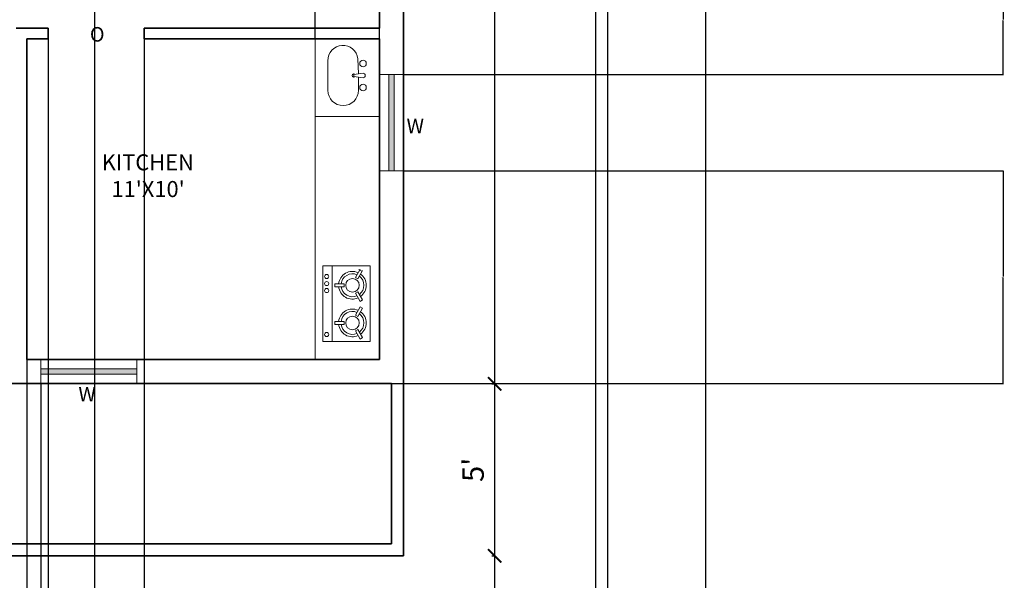
# Model space of a CAD drawing. Units: inches. Extents: x 502 to 1235, y -850 to 110.
# Tile 3 of 9: x 867 to 1235, y -625 to -415. Entities that reach past the tile are written whole.
import ezdxf

# ---------------------------------------------------------------- set-up
doc = ezdxf.new("R2010")
doc.units = ezdxf.units.IN
doc.header["$MEASUREMENT"] = 0
for name, color, linetype, lineweight in [('A-ANNO-DIMS', 2, 'Continuous', 18), ('A-ANNO-TEXT', 7, 'Continuous', 18), ('A-AREA-IDEN', 8, 'Continuous', 18), ('A-EQPM', 50, 'Continuous', 18), ('A-FLOR-CASE', 50, 'Continuous', 18), ('A-FLOR-FIXT', 50, 'Continuous', 18), ('A-GLAZ-PATT', 5, 'Continuous', 13), ('C-PROP', 1, 'Continuous', 25), ('WALL', 1, 'Continuous', 35), ('WIN', 5, 'Continuous', 18)]:
    doc.layers.add(name, color=color, linetype=linetype, lineweight=lineweight)
doc.styles.get("Standard").update_dxf_attribs({"font": 'arial.ttf'})
doc.dimstyles.get("Standard").update_dxf_attribs({"dimtxt": 0.18, "dimasz": 0.18, "dimexe": 0.18, "dimexo": 0.0625, "dimgap": 0.09, "dimtad": 0, "dimtih": 1, "dimtoh": 1, "dimdec": 1, "dimzin": 0, "dimdsep": 46, "dimlunit": 4, "dimtxsty": 'Standard', "dimcen": 0.09, "dimadec": 0, "dimazin": 0, "dimtfac": 1, "dimtdec": 1, "dimtofl": 0, "dimtmove": 0, "dimatfit": 3, "dimfxl": 1, "dimtolj": 1, "dimtzin": 0, "dimarcsym": 0})

# ---------------------------------------------------------------- blocks, each defined once
blk = doc.blocks.new('_ArchTick')
at = {"color": 0, "linetype": 'ByBlock', "const_width": 0.15}
blk.add_lwpolyline([(-0.5, -0.5), (0.5, 0.5)], dxfattribs=at)
blk = doc.blocks.new('*D6')
at = {"layer": 'A-ANNO-DIMS', "color": 0, "lineweight": -2, "transparency": 16777216}
for p, q in [((1122.49, 15.65), (1123.67, 15.65)), ((1123.49, 15.65), (1123.49, -704.35)), ((1122.49, -704.35), (1123.67, -704.35))]:
    blk.add_line(p, q, dxfattribs=at)
at = {"layer": 'Defpoints', "color": 0, "transparency": 16777216}
for p in [(1086.89, 15.65), (1086.89, -704.35), (1123.49, -704.35)]:
    blk.add_point(p, dxfattribs=at)
at = {"layer": 'A-ANNO-DIMS', "color": 0, "lineweight": -2, "transparency": 16777216, "xscale": 5, "yscale": 5, "zscale": 5}
for p, rotation in [((1123.49, 15.65), 90), ((1123.49, -704.35), 270)]:
    blk.add_blockref('_ArchTick', p, dxfattribs=dict(at, rotation=rotation))
at = {"layer": 'A-ANNO-DIMS', "color": 0, "transparency": 16777216, "insert": (1115.41, -344.35), "char_height": 8, "attachment_point": 5, "rotation": 90}
blk.add_mtext("\\A1;60'", dxfattribs=at)
blk = doc.blocks.new('*D7')
at = {"layer": 'A-ANNO-DIMS', "color": 0, "lineweight": -2, "transparency": 16777216}
for p, q in [((1043.54, -60.85), (1044.72, -60.85)), ((1044.54, -60.85), (1044.54, -551.48)), ((1043.54, -551.48), (1044.72, -551.48))]:
    blk.add_line(p, q, dxfattribs=at)
at = {"layer": 'Defpoints', "color": 0, "transparency": 16777216}
for p in [(1010.39, -60.85), (1010.39, -551.48), (1044.54, -551.48)]:
    blk.add_point(p, dxfattribs=at)
at = {"layer": 'A-ANNO-DIMS', "color": 0, "lineweight": -2, "transparency": 16777216, "xscale": 5, "yscale": 5, "zscale": 5}
for p, rotation in [((1044.54, -60.85), 90), ((1044.54, -551.48), 270)]:
    blk.add_blockref('_ArchTick', p, dxfattribs=dict(at, rotation=rotation))
at = {"layer": 'A-ANNO-DIMS', "color": 0, "transparency": 16777216, "insert": (1036.52, -306.16), "char_height": 8, "attachment_point": 5, "rotation": 90}
blk.add_mtext("\\A1;42'", dxfattribs=at)
blk = doc.blocks.new('*D8')
at = {"layer": 'A-ANNO-DIMS', "color": 0, "lineweight": -2, "transparency": 16777216}
for p, q in [((1043.54, -551.48), (1044.72, -551.48)), ((1044.54, -551.48), (1044.54, -615.85)), ((1043.54, -615.85), (1044.72, -615.85))]:
    blk.add_line(p, q, dxfattribs=at)
at = {"layer": 'Defpoints', "color": 0, "transparency": 16777216}
for p in [(1010.39, -551.48), (1010.39, -615.85), (1044.54, -615.85)]:
    blk.add_point(p, dxfattribs=at)
at = {"layer": 'A-ANNO-DIMS', "color": 0, "lineweight": -2, "transparency": 16777216, "xscale": 5, "yscale": 5, "zscale": 5}
for p, rotation in [((1044.54, -551.48), 90), ((1044.54, -615.85), 270)]:
    blk.add_blockref('_ArchTick', p, dxfattribs=dict(at, rotation=rotation))
at = {"layer": 'A-ANNO-DIMS', "color": 0, "transparency": 16777216, "insert": (1036.47, -583.66), "char_height": 8, "attachment_point": 5, "rotation": 90}
blk.add_mtext("\\A1;5'", dxfattribs=at)
blk = doc.blocks.new('*D9')
at = {"layer": 'A-ANNO-DIMS', "color": 0, "lineweight": -2, "transparency": 16777216}
for p, q in [((1043.54, -615.85), (1044.72, -615.85)), ((1044.54, -615.85), (1044.54, -699.85)), ((1043.54, -699.85), (1044.72, -699.85))]:
    blk.add_line(p, q, dxfattribs=at)
at = {"layer": 'Defpoints', "color": 0, "transparency": 16777216}
for p in [(1010.39, -615.85), (1012.7, -699.85), (1044.54, -699.85)]:
    blk.add_point(p, dxfattribs=at)
at = {"layer": 'A-ANNO-DIMS', "color": 0, "lineweight": -2, "transparency": 16777216, "xscale": 5, "yscale": 5, "zscale": 5}
for p, rotation in [((1044.54, -615.85), 90), ((1044.54, -699.85), 270)]:
    blk.add_blockref('_ArchTick', p, dxfattribs=dict(at, rotation=rotation))
at = {"layer": 'A-ANNO-DIMS', "color": 0, "transparency": 16777216, "insert": (1036.54, -657.85), "char_height": 8, "attachment_point": 5, "rotation": 90}
blk.add_mtext("\\A1;7'", dxfattribs=at)
blk = doc.blocks.new('WIN-36IN')
for p, q in [((0, 0), (0, 9)), ((36, 0), (36, 9)), ((0, 5.5), (36, 5.5)), ((0, 3.5), (36, 3.5))]:
    blk.add_line(p, q)
blk = doc.blocks.new('*D25')
at = {"layer": 'A-ANNO-DIMS', "color": 0, "lineweight": -2, "transparency": 16777216}
for p, q in [((798.89, -699.78), (798.89, 63.98)), ((799.07, 63.8), (846.56, 63.8)), ((894.71, 63.8), (847.22, 63.8)), ((894.89, -699.78), (894.89, 63.98))]:
    blk.add_line(p, q, dxfattribs=at)
at = {"layer": 'A-ANNO-DIMS', "color": 0, "transparency": 16777216}
for points in [[(799.07, 63.83), (799.07, 63.77), (798.89, 63.8)], [(894.71, 63.83), (894.71, 63.77), (894.89, 63.8)]]:
    blk.add_solid(points, dxfattribs=at)
at = {"layer": 'Defpoints', "color": 0, "transparency": 16777216}
for p in [(894.89, 63.8), (798.89, -699.85), (894.89, -699.85)]:
    blk.add_point(p, dxfattribs=at)
at = {"layer": 'A-ANNO-DIMS', "color": 0, "transparency": 16777216, "insert": (846.89, 63.8), "char_height": 0.18, "attachment_point": 5}
blk.add_mtext('\\A1;8\'-0"', dxfattribs=at)
blk = doc.blocks.new('*D41')
at = {"layer": 'A-ANNO-DIMS', "color": 0, "lineweight": -2, "transparency": 16777216}
for p, q in [((877.39, -422.41), (877.39, -844.7)), ((913.39, -422.41), (913.39, -844.7)), ((877.57, -844.52), (895.06, -844.52)), ((913.21, -844.52), (895.72, -844.52))]:
    blk.add_line(p, q, dxfattribs=at)
at = {"layer": 'A-ANNO-DIMS', "color": 0, "transparency": 16777216}
for points in [[(877.57, -844.49), (877.57, -844.55), (877.39, -844.52)], [(913.21, -844.49), (913.21, -844.55), (913.39, -844.52)]]:
    blk.add_solid(points, dxfattribs=at)
at = {"layer": 'Defpoints', "color": 0, "transparency": 16777216}
for p in [(877.39, -422.35), (913.39, -422.35), (913.39, -844.52)]:
    blk.add_point(p, dxfattribs=at)
at = {"layer": 'A-ANNO-DIMS', "color": 0, "transparency": 16777216, "insert": (895.39, -844.52), "char_height": 0.18, "attachment_point": 5}
blk.add_mtext('\\A1;3\'-0"', dxfattribs=at)
blk = doc.blocks.new('*D42')
at = {"layer": 'A-ANNO-DIMS', "color": 0, "lineweight": -2, "transparency": 16777216}
for p, q in [((869.39, -422.41), (869.39, -844.7)), ((877.39, -422.41), (877.39, -844.7)), ((869.57, -844.52), (873.06, -844.52)), ((877.21, -844.52), (873.72, -844.52))]:
    blk.add_line(p, q, dxfattribs=at)
at = {"layer": 'A-ANNO-DIMS', "color": 0, "transparency": 16777216}
for points in [[(869.57, -844.49), (869.57, -844.55), (869.39, -844.52)], [(877.21, -844.49), (877.21, -844.55), (877.39, -844.52)]]:
    blk.add_solid(points, dxfattribs=at)
at = {"layer": 'Defpoints', "color": 0, "transparency": 16777216}
for p in [(869.39, -422.35), (877.39, -422.35), (877.39, -844.52)]:
    blk.add_point(p, dxfattribs=at)
at = {"layer": 'A-ANNO-DIMS', "color": 0, "transparency": 16777216, "insert": (873.39, -844.52), "char_height": 0.18, "attachment_point": 5}
blk.add_mtext('\\A1;0\'-8"', dxfattribs=at)
blk = doc.blocks.new('*D43')
at = {"layer": 'A-ANNO-DIMS', "color": 0, "lineweight": -2, "transparency": 16777216}
for p, q in [((977.39, -422.28), (977.39, 63.98)), ((977.57, 63.8), (989.06, 63.8)), ((1001.21, 63.8), (989.72, 63.8)), ((1001.39, -422.28), (1001.39, 63.98))]:
    blk.add_line(p, q, dxfattribs=at)
at = {"layer": 'A-ANNO-DIMS', "color": 0, "transparency": 16777216}
for points in [[(977.57, 63.83), (977.57, 63.77), (977.39, 63.8)], [(1001.21, 63.83), (1001.21, 63.77), (1001.39, 63.8)]]:
    blk.add_solid(points, dxfattribs=at)
at = {"layer": 'Defpoints', "color": 0, "transparency": 16777216}
for p in [(1001.39, 63.8), (977.39, -422.35), (1001.39, -422.35)]:
    blk.add_point(p, dxfattribs=at)
at = {"layer": 'A-ANNO-DIMS', "color": 0, "transparency": 16777216, "insert": (989.39, 63.8), "char_height": 0.18, "attachment_point": 5}
blk.add_mtext('\\A1;2\'-0"', dxfattribs=at)
blk = doc.blocks.new('*D47')
at = {"layer": 'A-ANNO-DIMS', "color": 0, "lineweight": -2, "transparency": 16777216}
for p, q in [((857.39, -551.41), (857.39, -844.7)), ((874.64, -551.41), (874.64, -844.7)), ((857.57, -844.52), (865.69, -844.52)), ((874.46, -844.52), (866.34, -844.52))]:
    blk.add_line(p, q, dxfattribs=at)
at = {"layer": 'A-ANNO-DIMS', "color": 0, "transparency": 16777216}
for points in [[(857.57, -844.49), (857.57, -844.55), (857.39, -844.52)], [(874.46, -844.49), (874.46, -844.55), (874.64, -844.52)]]:
    blk.add_solid(points, dxfattribs=at)
at = {"layer": 'Defpoints', "color": 0, "transparency": 16777216}
for p in [(857.39, -551.35), (874.64, -551.35), (874.64, -844.52)]:
    blk.add_point(p, dxfattribs=at)
at = {"layer": 'A-ANNO-DIMS', "color": 0, "transparency": 16777216, "insert": (866.01, -844.52), "char_height": 0.18, "attachment_point": 5}
blk.add_mtext('\\A1;1\'-5"', dxfattribs=at)
blk = doc.blocks.new('*D54')
at = {"layer": 'A-ANNO-DIMS', "color": 0, "lineweight": -2, "transparency": 16777216}
for p, q in [((1010.45, -471.74), (1235.01, -471.74)), ((1234.83, -471.92), (1234.83, -511.36)), ((1234.83, -551.17), (1234.83, -511.73)), ((1005.95, -551.35), (1235.01, -551.35))]:
    blk.add_line(p, q, dxfattribs=at)
at = {"layer": 'A-ANNO-DIMS', "color": 0, "transparency": 16777216}
for points in [[(1234.8, -471.92), (1234.86, -471.92), (1234.83, -471.74)], [(1234.8, -551.17), (1234.86, -551.17), (1234.83, -551.35)]]:
    blk.add_solid(points, dxfattribs=at)
at = {"layer": 'Defpoints', "color": 0, "transparency": 16777216}
for p in [(1010.39, -471.74), (1234.83, -471.74), (1005.89, -551.35)]:
    blk.add_point(p, dxfattribs=at)
at = {"layer": 'A-ANNO-DIMS', "color": 0, "transparency": 16777216, "insert": (1234.83, -511.54), "char_height": 0.18, "attachment_point": 5}
blk.add_mtext('\\A1;6\'-7 1/2"', dxfattribs=at)
blk = doc.blocks.new('*D55')
at = {"layer": 'A-ANNO-DIMS', "color": 0, "lineweight": -2, "transparency": 16777216}
for p, q in [((1010.45, -394.85), (1235.01, -394.85)), ((1234.83, -395.03), (1234.83, -415.12)), ((1234.83, -435.56), (1234.83, -415.48)), ((1010.45, -435.74), (1235.01, -435.74))]:
    blk.add_line(p, q, dxfattribs=at)
at = {"layer": 'A-ANNO-DIMS', "color": 0, "transparency": 16777216}
for points in [[(1234.8, -395.03), (1234.86, -395.03), (1234.83, -394.85)], [(1234.8, -435.56), (1234.86, -435.56), (1234.83, -435.74)]]:
    blk.add_solid(points, dxfattribs=at)
at = {"layer": 'Defpoints', "color": 0, "transparency": 16777216}
for p in [(1010.39, -394.85), (1234.83, -394.85), (1010.39, -435.74)]:
    blk.add_point(p, dxfattribs=at)
at = {"layer": 'A-ANNO-DIMS', "color": 0, "transparency": 16777216, "insert": (1234.83, -415.3), "char_height": 0.18, "attachment_point": 5}
blk.add_mtext('\\A1;3\'-5"', dxfattribs=at)

msp = doc.modelspace()

# ---------------------------------------------------------------- hatches: boundary and pattern name
at = {"layer": 'A-GLAZ-PATT'}
h = msp.add_hatch(color=256, dxfattribs=at)
h.dxf.hatch_style = 1
h.paths.add_polyline_path([(769.5, -64.35), (769.5, -66.35), (805.5, -66.35), (805.5, -64.35)])
h.paths.add_polyline_path([(845.65, -64.35), (821.65, -64.35), (821.65, -66.35), (845.65, -66.35)])
h.paths.add_polyline_path([(995.07, -64.35), (959.07, -64.35), (959.07, -66.35), (995.07, -66.35)])
h.paths.add_polyline_path([(1006.89, -358.85), (1004.89, -358.85), (1004.89, -394.85), (1006.89, -394.85)])
h.paths.add_polyline_path([(1006.89, -435.74), (1004.89, -435.74), (1004.89, -471.74), (1006.89, -471.74)])
h.paths.add_polyline_path([(874.64, -545.85), (874.64, -547.85), (910.64, -547.85), (910.64, -545.85)])
h.paths.add_polyline_path([(640.89, -310.35), (638.89, -310.35), (638.89, -334.35), (640.89, -334.35)])
h.paths.add_polyline_path([(640.89, -358.06), (638.89, -358.06), (638.89, -394.06), (640.89, -394.06)])

# ---------------------------------------------------------------- linework, layer by layer
at = {"layer": 'A-EQPM'}
for p, q in [((980.22, -535.62), (980.22, -507.27)), ((980.22, -507.27), (997.94, -507.27)), ((983.77, -535.62), (983.77, -507.27)), ((997.94, -535.62), (997.94, -507.27)), ((992.41, -511.65), (994.17, -508.59)), ((992.41, -511.65), (993.33, -512.18)), ((993.33, -512.18), (995.09, -509.12)), ((993.76, -508.73), (994.78, -509.32)), ((988.21, -514.07), (984.68, -514.06)), ((984.68, -515.13), (984.68, -514.06)), ((988.21, -515.13), (984.68, -515.13)), ((988.21, -515.13), (988.21, -514.07)), ((993.32, -517.02), (992.4, -517.55)), ((992.4, -517.55), (994.17, -520.61)), ((993.32, -517.02), (995.09, -520.08)), ((992.41, -525.73), (994.17, -522.68)), ((993.33, -526.27), (995.09, -523.21)), ((995.09, -520.08), (994.17, -520.61)), ((994.17, -522.68), (995.09, -523.21)), ((992.41, -525.73), (993.33, -526.27)), ((988.21, -528.15), (984.68, -528.15)), ((984.68, -529.22), (984.68, -528.15)), ((988.21, -529.22), (984.68, -529.22)), ((988.21, -529.22), (988.21, -528.15)), ((993.32, -531.11), (992.4, -531.64)), ((992.4, -531.64), (994.17, -534.7)), ((993.32, -531.11), (995.09, -534.17)), ((995.09, -534.17), (994.17, -534.7)), ((980.22, -535.62), (997.94, -535.62))]:
    msp.add_line(p, q, dxfattribs=at)
at = {"layer": 'A-EQPM', "extrusion": (0, 0, -1)}
for centre, major_axis, start_param, end_param in [((981.68, -511.31), (0.544, 0.544), 2.35619449019219, 8.639379797371777), ((991.31, -514.6), (5.19, 0), 3.2451, 5.134376), ((991.31, -514.6), (3.04, 3.04), 4.051123, 5.898002), ((991.31, -514.6), (1.79, 1.79), 2.356194490192312, 8.639379797371898), ((991.31, -514.6), (3.04, 3.04), 6.145519, 7.992397), ((991.31, -514.6), (5.19, 0.01), -0.942584, 0.946692), ((981.68, -513.97), (0.544, 0.544), 2.35619449019219, 8.639379797371777), ((981.68, -516.57), (0.544, 0.544), 2.35619449019219, 8.639379797371777), ((991.31, -514.6), (5.19, -0.01), 1.148752, 3.038029), ((991.31, -514.6), (3.04, -3.04), 0.385932, 2.23281), ((991.31, -528.69), (5.19, 0), 3.244173, 5.13345), ((991.31, -528.69), (3.04, -3.04), 2.480327, 4.327205), ((991.31, -528.69), (1.79, 1.79), 2.356194490192306, 8.639379797371893), ((991.31, -528.69), (3.04, 3.04), 6.145519, 7.992397), ((991.31, -528.69), (5.19, 0), -0.944011, 0.945266), ((991.31, -528.69), (5.19, -0.01), 1.14879, 3.038067), ((991.31, -528.69), (3.04, -3.04), 0.385932, 2.23281), ((981.68, -533.03), (0.544, 0.544), 2.35619449019219, 8.639379797371777)]:
    msp.add_ellipse(centre, major_axis=major_axis, ratio=1, start_param=start_param, end_param=end_param, dxfattribs=at)
at = {"layer": 'A-FLOR-CASE'}
for p, q in [((977.39, -542.35), (977.39, -422.35)), ((977.34, -451.48), (1001.34, -451.48))]:
    msp.add_line(p, q, dxfattribs=at)
at = {"layer": 'A-FLOR-FIXT'}
for p, q in [((982.1, -430.56), (982.1, -441.62)), ((993.37, -429.84), (993.53, -435.48)), ((991.78, -435.68), (995.27, -435.27)), ((991.78, -436.56), (991.78, -435.68)), ((995.27, -436.91), (991.78, -436.5)), ((993.57, -436.71), (993.57, -441.62))]:
    msp.add_line(p, q, dxfattribs=at)
for centre in [(995.27, -431.58), (995.27, -440.6)]:
    msp.add_circle(centre, 1.23, dxfattribs=at)
for centre, radius, start, end in [((987.75, -430.47), 5.65, 6.3659, 180.8792), ((991.78, -436.09), 0.615, 48.1701, 311.8299), ((995.27, -436.09), 0.82, 270, 90), ((987.84, -441.62), 5.74, 180, 0)]:
    msp.add_arc(centre, radius, start, end, dxfattribs=at)
at = {"layer": 'C-PROP'}
for p, q in [((1086.89, -704.35), (1086.89, 15.65)), ((1082.39, -699.85), (1082.39, 11.15))]:
    msp.add_line(p, q, dxfattribs=at)
at = {"layer": 'WALL'}
for p, q in [((1010.39, -615.85), (1010.39, -60.85)), ((1001.39, -418.35), (1001.39, -193.85)), ((865.39, -418.35), (877.39, -418.35)), ((877.39, -422.35), (877.39, -418.35)), ((913.39, -422.35), (913.39, -418.35)), ((913.39, -418.35), (1001.39, -418.35)), ((869.39, -542.35), (869.39, -422.35)), ((869.39, -422.35), (877.39, -422.35)), ((913.39, -422.35), (1001.39, -422.35)), ((1001.39, -542.35), (1001.39, -422.35)), ((869.39, -542.35), (1001.39, -542.35)), ((857.39, -551.35), (1005.89, -551.35)), ((1005.89, -611.35), (1005.89, -551.35)), ((639.89, -611.35), (1005.89, -611.35)), ((635.39, -615.85), (1010.39, -615.85))]:
    msp.add_line(p, q, dxfattribs=at)

# ---------------------------------------------------------------- block references
at = {"layer": 'WIN', "rotation": 269.9999999999997}
msp.add_blockref('WIN-36IN', (1001.39, -435.74), dxfattribs=at)
at = {"layer": 'WIN'}
msp.add_blockref('WIN-36IN', (874.64, -551.35), dxfattribs=at)

# ---------------------------------------------------------------- texts
at = {"layer": 'A-ANNO-TEXT'}
for s, p in [('O', (893.04, -423.41)), ('W', (1011.57, -457.69)), ('W', (888.74, -558.06))]:
    msp.add_text(s, height=5.44, dxfattribs=at).set_placement(p)
at = {"layer": 'A-AREA-IDEN', "insert": (890.12, -465.59), "char_height": 6, "attachment_point": 1}
msp.add_mtext_dynamic_manual_height_columns("    KITCHEN\\P      11'X10'", width=53.3957, gutter_width=1, heights=[0], dxfattribs=at)

# ---------------------------------------------------------------- dimensions: what is measured, and where the dimension line sits
at = {"layer": 'A-ANNO-DIMS'}
for base, p1, p2, picture, middle in [((894.89, 63.8), (798.89, -699.85), (894.89, -699.85), '*D25', (846.89, 63.8)), ((1001.39, 63.8), (977.39, -422.35), (1001.39, -422.35), '*D43', (989.39, 63.8)), ((877.39, -844.52), (869.39, -422.35), (877.39, -422.35), '*D42', (873.39, -844.52)), ((913.39, -844.52), (877.39, -422.35), (913.39, -422.35), '*D41', (895.39, -844.52)), ((874.6386, -844.5172), (857.3902, -551.3456), (874.6386, -551.3456), '*D47', (866.0144, -844.5172))]:
    dim = msp.add_linear_dim(base=base, p1=p1, p2=p2, dimstyle='Standard', override={"dimdec": 1, "dimlfac": 1, "dimrnd": 0, "dimzin": 1, "dimdsep": 46, "dimlunit": 4, "dimfrac": 2}, dxfattribs=at)
    dim.commit()
    dim.dimension.update_dxf_attribs({"geometry": picture, "text_midpoint": middle})
for base, p1, p2, override, picture, middle in [((1123.49, -704.35), (1086.89, 15.65), (1086.89, -704.35), {"dimtxt": 8, "dimasz": 5, "dimgap": 4, "dimtad": 1, "dimtih": 0, "dimblk1": 'ArchTick', "dimblk2": 'ArchTick', "dimsah": 1, "dimclrd": 0, "dimclre": 0, "dimclrt": 0, "dimfxlon": 1}, '*D6', (1115.41, -344.35)), ((1234.83, -394.85), (1010.39, -435.74), (1010.39, -394.85), {"dimdec": 1, "dimlfac": 1, "dimrnd": 0, "dimzin": 1, "dimdsep": 46, "dimlunit": 4, "dimfrac": 2}, '*D55', (1234.83, -415.3)), ((1234.83, -471.74), (1005.89, -551.35), (1010.39, -471.74), {"dimdec": 1, "dimlfac": 1, "dimrnd": 0, "dimzin": 1, "dimdsep": 46, "dimlunit": 4, "dimfrac": 2}, '*D54', (1234.83, -511.54)), ((1044.54, -699.85), (1010.39, -615.85), (1012.7, -699.85), {"dimtxt": 8, "dimasz": 5, "dimgap": 4, "dimtad": 1, "dimtih": 0, "dimblk1": 'ArchTick', "dimblk2": 'ArchTick', "dimsah": 1, "dimclrd": 0, "dimclre": 0, "dimclrt": 0, "dimfxlon": 1}, '*D9', (1036.54, -657.85))]:
    dim = msp.add_linear_dim(base=base, p1=p1, p2=p2, angle=90, dimstyle='Standard', override=override, dxfattribs=at)
    dim.commit()
    dim.dimension.update_dxf_attribs({"geometry": picture, "text_midpoint": middle})
for base, p1, p2, text, picture, middle in [((1044.54, -551.48), (1010.39, -60.85), (1010.39, -551.48), "42'", '*D7', (1036.52, -306.16)), ((1044.54, -615.85), (1010.39, -551.48), (1010.39, -615.85), "5'", '*D8', (1036.47, -583.66))]:
    dim = msp.add_linear_dim(base=base, p1=p1, p2=p2, angle=90, text=text, dimstyle='Standard', override={"dimtxt": 8, "dimasz": 5, "dimgap": 4, "dimtad": 1, "dimtih": 0, "dimblk1": 'ArchTick', "dimblk2": 'ArchTick', "dimsah": 1, "dimclrd": 0, "dimclre": 0, "dimclrt": 0, "dimfxlon": 1}, dxfattribs=at)
    dim.commit()
    dim.dimension.update_dxf_attribs({"geometry": picture, "text_midpoint": middle})

doc.saveas('drawing.dxf')
